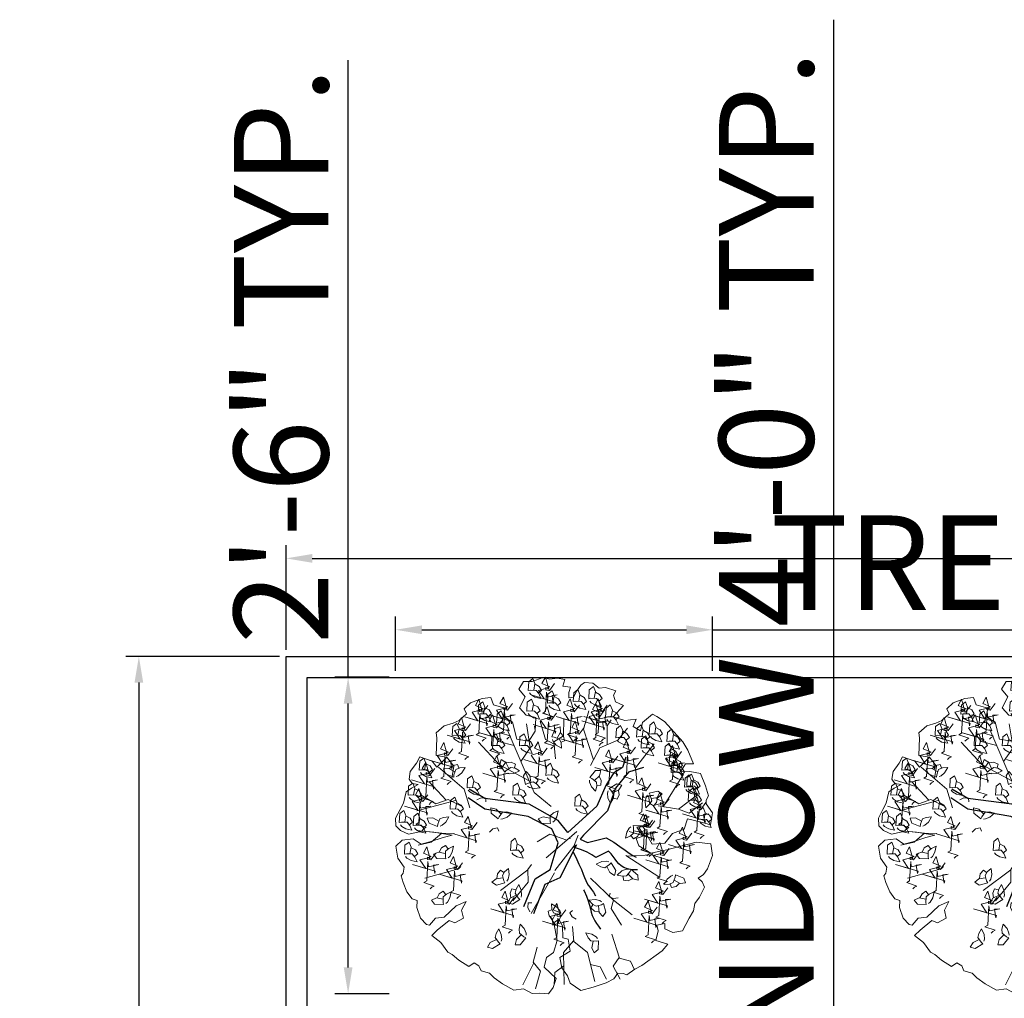
# Model space of a CAD drawing. Units: inches. Extents: x 2831 to 4250, y 1103 to 1797.
# Tile 4 of 15: x 3418 to 3512, y 1690 to 1783. Entities that reach past the tile are written whole.
import ezdxf

# ---------------------------------------------------------------- set-up
doc = ezdxf.new("R2010")
doc.units = ezdxf.units.IN
for name, color, linetype, lineweight in [('A-ANNO-DIMS', 2, 'Continuous', 18), ('ARBOL', 30, 'Continuous', 13), ('C-PROP', 7, 'Continuous', 25)]:
    doc.layers.add(name, color=color, linetype=linetype, lineweight=lineweight)
doc.layers.add('TALLO', color=36, linetype='Continuous')
doc.styles.get("Standard").update_dxf_attribs({"font": 'arial.ttf'})
doc.dimstyles.new('ISO-25', dxfattribs={"dimtxt": 9, "dimasz": 2.5, "dimexe": 1.25, "dimexo": 0.625, "dimtad": 1, "dimdec": 1, "dimlunit": 3, "dimtxsty": 'Standard', "dimcen": 2.5, "dimadec": 0, "dimazin": 0, "dimtfac": 1, "dimtdec": 1, "dimtmove": 0, "dimatfit": 3, "dimfxl": 1, "dimarcsym": 0})

# ---------------------------------------------------------------- blocks, each defined once
blk = doc.blocks.new('*D5')
at = {"layer": 'A-ANNO-DIMS', "color": 0, "lineweight": -2, "transparency": 16777216}
for p, q in [((3443.227, 1723.138), (3443.227, 1733.099)), ((3803.227, 1723.138), (3803.227, 1733.099)), ((3445.727, 1731.849), (3800.727, 1731.849))]:
    blk.add_line(p, q, dxfattribs=at)
at = {"layer": 'A-ANNO-DIMS', "color": 0, "transparency": 16777216}
for points in [[(3445.727, 1732.265), (3445.727, 1731.432), (3443.227, 1731.849)], [(3800.727, 1732.265), (3800.727, 1731.432), (3803.227, 1731.849)]]:
    blk.add_solid(points, dxfattribs=at)
at = {"layer": 'Defpoints', "color": 0, "transparency": 16777216}
for p in [(3803.227, 1731.849), (3443.227, 1722.513), (3803.227, 1722.513)]:
    blk.add_point(p, dxfattribs=at)
at = {"layer": 'A-ANNO-DIMS', "color": 0, "transparency": 16777216, "insert": (3623.227, 1737.072), "char_height": 9, "attachment_point": 5}
blk.add_mtext("30'", dxfattribs=at)
blk = doc.blocks.new('*D6')
at = {"layer": 'A-ANNO-DIMS', "color": 0, "lineweight": -2, "transparency": 16777216}
for p, q in [((3442.602, 1722.513), (3427.958, 1722.513)), ((3429.208, 1720.013), (3429.208, 1245.013)), ((3442.602, 1242.513), (3427.958, 1242.513))]:
    blk.add_line(p, q, dxfattribs=at)
at = {"layer": 'A-ANNO-DIMS', "color": 0, "transparency": 16777216}
for points in [[(3428.791, 1720.013), (3429.625, 1720.013), (3429.208, 1722.513)], [(3428.791, 1245.013), (3429.625, 1245.013), (3429.208, 1242.513)]]:
    blk.add_solid(points, dxfattribs=at)
at = {"layer": 'Defpoints', "color": 0, "transparency": 16777216}
for p in [(3443.227, 1722.513), (3429.208, 1242.513), (3443.227, 1242.513)]:
    blk.add_point(p, dxfattribs=at)
at = {"layer": 'A-ANNO-DIMS', "color": 0, "transparency": 16777216, "insert": (3423.988, 1482.513), "char_height": 9, "attachment_point": 5, "rotation": 90}
blk.add_mtext("40'", dxfattribs=at)
blk = doc.blocks.new('fresno')
at = {"layer": 'ARBOL'}
for p, q in [((2.96, 0.991), (3.575, 1.984)), ((-3.638, 1.194), (-4.164, 1.76)), ((-1.151, -0.932), (-1.99, -1.556)), ((-0.974, -3.757), (-1.31, -4.423))]:
    blk.add_line(p, q, dxfattribs=at)
blk.add_lwpolyline([(0.823, 4.745), (0.566, 4.764), (0.459, 4.687), (0.336, 4.518), (0.233, 4.322), (0.087, 4.298), (0.091, 4.464), (0.14, 4.621), (-0.09, 4.659), (-0.033, 4.863), (-0.264, 4.901), (-0.483, 4.866), (-0.686, 4.924), (-1.021, 4.801), (-1.288, 4.8), (-1.431, 4.563), (-1.234, 4.327), (-1.406, 4), (-1.205, 3.778), (-0.909, 3.705), (-0.931, 3.283), (-1.122, 2.983), (-1.491, 3.043), (-1.619, 3.562), (-1.9, 3.727), (-1.851, 3.982), (-2.197, 4.084), (-2.278, 4.31), (-2.543, 4.283), (-2.896, 4.152), (-3.091, 3.971), (-3.022, 3.817), (-3.244, 3.617), (-3.424, 3.528), (-3.697, 3.455), (-3.946, 3.236), (-3.922, 3.09), (-3.94, 2.548), (-3.617, 2.495), (-3.927, 2.19), (-4.062, 2.379), (-4.443, 2.512), (-4.546, 2.316), (-4.73, 2.062), (-4.767, 1.832), (-4.671, 1.698), (-4.486, 1.667), (-4.693, 1.559), (-4.854, 1.444), (-4.934, 1.102), (-5.037, 0.905), (-5.175, 0.644), (-5.166, 0.406), (-5.024, 0.264), (-4.781, 0.153), (-4.363, 0.249), (-4.014, 0.215), (-3.783, 0.177), (-3.46, 0.124), (-3.733, 0.051), (-4.132, -0.073), (-4.404, -0.146), (-4.639, 0.011), (-4.977, -0.028), (-5.172, -0.209), (-5.113, -0.574), (-4.921, -0.843), (-4.951, -1.027), (-5.012, -1.112), (-4.95, -1.311), (-4.83, -1.592), (-4.676, -1.807), (-4.518, -1.856), (-4.529, -2.068), (-4.417, -2.394), (-4.236, -2.59), (-4.143, -2.605), (-3.967, -2.397), (-3.703, -2.37), (-3.339, -2.027), (-3.032, -1.889), (-3.169, -2.15), (-3.115, -2.396), (-3.376, -2.542), (-3.552, -2.466), (-3.909, -2.762), (-4.077, -2.924), (-3.804, -3.135), (-3.592, -3.43), (-3.461, -3.499), (-3.253, -3.676), (-2.953, -3.867), (-2.792, -3.752), (-2.642, -3.848), (-2.572, -4.001), (-2.323, -4.066), (-2.18, -4.208), (-1.926, -4.392), (-1.58, -4.591), (-1.288, -4.545), (-1.027, -4.683), (-0.788, -4.675), (-0.531, -4.693), (-0.382, -4.505), (-0.29, -4.236), (-0.66, -3.891), (-0.588, -3.595), (-0.374, -3.441), (-0.267, -3.079), (-0.368, -2.541), (-0.208, -2.426), (-0.099, -2.633), (-0.087, -2.991), (0.071, -3.04), (0.129, -3.405), (-0.185, -3.59), (-0.119, -3.909), (0.055, -4.151), (0.136, -4.377), (0.456, -4.596), (0.828, -4.491), (1.227, -4.368), (1.461, -4.241), (1.583, -4.071), (1.748, -4.075), (1.86, -4.117), (2.101, -3.944), (2.308, -3.836), (2.925, -3.393), (3.101, -3.185), (2.74, -3.078), (2.812, -2.782), (2.769, -2.61), (3.015, -2.555), (3.012, -2.721), (3.254, -2.832), (3.546, -2.785), (3.752, -2.393), (3.882, -2.177), (3.92, -1.947), (4.069, -1.758), (4.214, -1.451), (4.144, -1.297), (4.021, -1.182), (4.182, -1.067), (4.304, -0.897), (4.464, -0.497), (4.429, -0.279), (4.406, -0.133), (3.964, -0.083), (3.074, -0.315), (2.582, -0.424), (2.217, -0.197), (2.136, 0.029), (2.462, 0.141), (2.628, -0.147), (3.012, -0.116), (3.249, 0.177), (3.602, 0.308), (3.701, 0.623), (4.089, 0.535), (4.404, 0.436), (4.464, 0.805), (4.272, 1.074), (4.267, 1.193), (4.336, 1.324), (4.243, 1.623), (4.092, 2.003), (3.769, 2.057), (3.485, 2.056), (3.642, 2.291), (3.88, 2.299), (3.71, 2.706), (3.563, 2.967), (3.201, 3.358), (3.001, 3.581), (2.766, 3.738), (2.635, 3.807), (2.332, 3.549), (2.268, 3.299), (2.052, 3.429), (2.136, 3.652), (1.798, 3.613), (1.437, 3.72), (1.755, 4.071), (1.513, 4.182), (1.451, 4.381), (1.519, 4.512), (1.204, 4.611), (1.012, 4.596)], close=True, dxfattribs=at)
for points in [[(-1.104, 4.45), (-1.063, 4.399), (-0.939, 4.325), (-0.757, 4.285), (-0.82, 4.431), (-0.903, 4.527), (-1.075, 4.533), (-1.143, 4.521), (-1.126, 4.792), (-1.002, 4.891), (-0.939, 4.738), (-0.975, 4.535)], [(-0.346, 4.735), (-0.501, 4.528), (-0.605, 4.545), (-0.605, 4.614), (-0.519, 4.563), (-0.622, 4.925), (-0.726, 4.735), (-0.484, 4.632), (-0.622, 4.58), (-0.829, 4.528), (-0.657, 4.27), (-1.053, 4.39), (-0.363, 4.183), (-0.381, 4.114), (-0.415, 4.373), (-0.26, 4.39), (-0.57, 4.321), (-0.588, 4.476), (-0.622, 3.89), (-0.708, 3.839), (-0.398, 3.735), (-0.467, 3.701), (-0.519, 3.649)], [(-0.935, 4.717), (-0.809, 4.65), (-0.736, 4.529), (-0.824, 4.459)], [(-0.521, 4.069), (-0.48, 4.018), (-0.356, 3.944), (-0.174, 3.904), (-0.237, 4.051), (-0.32, 4.146), (-0.492, 4.152), (-0.56, 4.14), (-0.543, 4.411), (-0.419, 4.511), (-0.356, 4.357), (-0.392, 4.154)], [(0.263, 4.114), (0.304, 4.063), (0.429, 3.989), (0.611, 3.948), (0.547, 4.095), (0.465, 4.191), (0.293, 4.197), (0.225, 4.185), (0.242, 4.456), (0.366, 4.555), (0.428, 4.402), (0.393, 4.199)], [(0.734, 4.203), (0.775, 4.152), (0.9, 4.078), (1.082, 4.038), (1.018, 4.185), (0.936, 4.281), (0.763, 4.287), (0.696, 4.274), (0.712, 4.546), (0.837, 4.645), (0.899, 4.491), (0.863, 4.289)], [(-2.368, 4.073), (-2.523, 3.866), (-2.627, 3.883), (-2.627, 3.952), (-2.541, 3.9), (-2.644, 4.262), (-2.748, 4.073), (-2.506, 3.969), (-2.644, 3.918), (-2.851, 3.866), (-2.679, 3.607), (-3.075, 3.728), (-2.385, 3.521), (-2.403, 3.452), (-2.437, 3.711), (-2.282, 3.728), (-2.592, 3.659), (-2.61, 3.814), (-2.644, 3.228), (-2.73, 3.176), (-2.42, 3.073), (-2.489, 3.038), (-2.541, 2.987)], [(-1.623, 4.132), (-1.778, 3.925), (-1.882, 3.942), (-1.882, 4.011), (-1.795, 3.959), (-1.899, 4.321), (-2.002, 4.132), (-1.761, 4.028), (-1.899, 3.977), (-2.106, 3.925), (-1.933, 3.666), (-2.33, 3.787), (-1.64, 3.58), (-1.657, 3.511), (-1.692, 3.77), (-1.537, 3.787), (-1.847, 3.718), (-1.864, 3.873), (-1.899, 3.287), (-1.985, 3.235), (-1.675, 3.132), (-1.744, 3.097), (-1.795, 3.046)], [(-1.149, 3.822), (-1.108, 3.771), (-0.983, 3.697), (-0.802, 3.657), (-0.865, 3.804), (-0.948, 3.9), (-1.12, 3.906), (-1.188, 3.893), (-1.171, 4.165), (-1.047, 4.264), (-0.984, 4.111), (-1.02, 3.908)], [(-0.352, 4.337), (-0.226, 4.269), (-0.153, 4.148), (-0.241, 4.078)], [(0.413, 4.08), (0.258, 3.873), (0.154, 3.89), (0.154, 3.959), (0.241, 3.908), (0.137, 4.27), (0.034, 4.08), (0.275, 3.977), (0.137, 3.925), (-0.07, 3.873), (0.103, 3.614), (-0.294, 3.735), (0.396, 3.528), (0.379, 3.459), (0.344, 3.718), (0.499, 3.735), (0.189, 3.666), (0.172, 3.821), (0.137, 3.235), (0.051, 3.183), (0.361, 3.08), (0.292, 3.046), (0.241, 2.994)], [(0.433, 4.381), (0.558, 4.314), (0.631, 4.193), (0.544, 4.122)], [(1.259, 4.08), (1.103, 3.873), (1, 3.89), (1, 3.959), (1.086, 3.908), (0.982, 4.27), (0.879, 4.08), (1.12, 3.977), (0.982, 3.925), (0.775, 3.873), (0.948, 3.614), (0.551, 3.735), (1.241, 3.528), (1.224, 3.459), (1.189, 3.718), (1.345, 3.735), (1.034, 3.666), (1.017, 3.821), (0.982, 3.235), (0.896, 3.183), (1.207, 3.08), (1.138, 3.046), (1.086, 2.994)], [(0.904, 4.471), (1.029, 4.404), (1.102, 4.282), (1.015, 4.212)], [(-2.629, 3.733), (-2.588, 3.682), (-2.463, 3.608), (-2.281, 3.568), (-2.345, 3.715), (-2.427, 3.81), (-2.6, 3.816), (-2.667, 3.804), (-2.651, 4.075), (-2.526, 4.175), (-2.464, 4.021), (-2.5, 3.818)], [(-2.459, 4), (-2.334, 3.933), (-2.261, 3.812), (-2.348, 3.742)], [(-2.068, 3.464), (-2.027, 3.413), (-1.903, 3.339), (-1.721, 3.299), (-1.784, 3.446), (-1.867, 3.542), (-2.039, 3.547), (-2.107, 3.535), (-2.09, 3.806), (-1.966, 3.906), (-1.903, 3.752), (-1.939, 3.55)], [(-0.287, 3.833), (-0.442, 3.626), (-0.546, 3.643), (-0.546, 3.712), (-0.46, 3.661), (-0.563, 4.023), (-0.667, 3.833), (-0.425, 3.73), (-0.563, 3.678), (-0.77, 3.626), (-0.598, 3.367), (-0.995, 3.488), (-0.304, 3.281), (-0.322, 3.212), (-0.356, 3.471), (-0.201, 3.488), (-0.511, 3.419), (-0.529, 3.574), (-0.563, 2.988), (-0.649, 2.936), (-0.339, 2.833), (-0.408, 2.799), (-0.46, 2.747)], [(-0.98, 4.09), (-0.854, 4.023), (-0.781, 3.901), (-0.869, 3.831)], [(1.189, 3.942), (1.034, 3.735), (0.931, 3.752), (0.931, 3.821), (1.017, 3.77), (0.913, 4.132), (0.81, 3.942), (1.051, 3.839), (0.913, 3.787), (0.706, 3.735), (0.879, 3.477), (0.482, 3.597), (1.172, 3.39), (1.155, 3.321), (1.12, 3.58), (1.276, 3.597), (0.965, 3.528), (0.948, 3.683), (0.913, 3.097), (0.827, 3.046), (1.138, 2.942), (1.069, 2.908), (1.017, 2.856)], [(0.837, 2.414), (0.533, 3.352), (0.697, 3.906)], [(1.25, 3.643), (1.291, 3.592), (1.416, 3.518), (1.597, 3.478), (1.534, 3.625), (1.451, 3.721), (1.279, 3.727), (1.211, 3.714), (1.228, 3.985), (1.352, 4.085), (1.415, 3.931), (1.379, 3.729)], [(1.419, 3.911), (1.545, 3.844), (1.618, 3.722), (1.53, 3.652)], [(-2.898, 3.511), (-3.053, 3.304), (-3.157, 3.321), (-3.157, 3.39), (-3.071, 3.339), (-3.174, 3.701), (-3.278, 3.511), (-3.036, 3.408), (-3.174, 3.356), (-3.381, 3.304), (-3.209, 3.046), (-3.605, 3.166), (-2.915, 2.959), (-2.932, 2.89), (-2.967, 3.149), (-2.812, 3.166), (-3.122, 3.097), (-3.14, 3.253), (-3.174, 2.666), (-3.26, 2.615), (-2.95, 2.511), (-3.019, 2.477), (-3.071, 2.425)], [(-1.951, 3.597), (-2.106, 3.39), (-2.209, 3.408), (-2.209, 3.477), (-2.123, 3.425), (-2.227, 3.787), (-2.33, 3.597), (-2.089, 3.494), (-2.227, 3.442), (-2.434, 3.39), (-2.261, 3.132), (-2.658, 3.252), (-1.968, 3.046), (-1.985, 2.977), (-2.02, 3.235), (-1.864, 3.252), (-2.175, 3.183), (-2.192, 3.339), (-2.227, 2.752), (-2.313, 2.701), (-2.002, 2.597), (-2.071, 2.563), (-2.123, 2.511)], [(-1.899, 3.732), (-1.773, 3.664), (-1.7, 3.543), (-1.788, 3.473)], [(-0.358, 2.895), (-0.615, 3.037), (-0.783, 3.596)], [(-0.063, 3.671), (-0.069, 3.151), (-0.364, 2.965), (-0.319, 2.449)], [(1.259, 2.882), (1.254, 3.446), (1.381, 3.636)], [(-3.413, 3.083), (-3.373, 3.032), (-3.248, 2.958), (-3.066, 2.918), (-3.129, 3.065), (-3.212, 3.161), (-3.384, 3.167), (-3.452, 3.154), (-3.435, 3.425), (-3.311, 3.525), (-3.248, 3.371), (-3.284, 3.169)], [(-3.244, 3.351), (-3.118, 3.284), (-3.045, 3.162), (-3.133, 3.092)], [(-0.448, 1), (-0.961, 1.419), (-1.784, 3.341)], [(-1.367, 2.367), (-1.081, 2.78), (-1.193, 3.514)], [(-0.923, 3.449), (-0.951, 3.425), (-0.93, 3.313)], [(-0.41, 3.035), (-0.387, 2.974), (-0.291, 2.865), (-0.131, 2.771), (-0.146, 2.93), (-0.195, 3.047), (-0.357, 3.106), (-0.425, 3.115), (-0.325, 3.368), (-0.176, 3.424), (-0.164, 3.258), (-0.261, 3.077)], [(0.558, 3.402), (0.403, 3.195), (0.299, 3.212), (0.299, 3.281), (0.386, 3.23), (0.282, 3.592), (0.179, 3.402), (0.42, 3.299), (0.282, 3.247), (0.075, 3.195), (0.248, 2.936), (-0.149, 3.057), (0.541, 2.85), (0.524, 2.781), (0.489, 3.04), (0.644, 3.057), (0.334, 2.988), (0.317, 3.143), (0.282, 2.557), (0.196, 2.505), (0.506, 2.402), (0.437, 2.368), (0.386, 2.316)], [(0.746, 2.242), (1.034, 2.786), (1.584, 3.019), (1.879, 3.374)], [(1.564, 3.016), (1.605, 2.965), (1.729, 2.891), (1.911, 2.851), (1.848, 2.998), (1.765, 3.094), (1.593, 3.099), (1.525, 3.087), (1.542, 3.358), (1.666, 3.458), (1.729, 3.304), (1.693, 3.102)], [(2.191, 3.038), (2.232, 2.987), (2.357, 2.913), (2.539, 2.873), (2.475, 3.02), (2.393, 3.116), (2.221, 3.122), (2.153, 3.109), (2.17, 3.381), (2.294, 3.48), (2.356, 3.326), (2.321, 3.124)], [(2.361, 3.306), (2.486, 3.239), (2.559, 3.117), (2.472, 3.047)], [(2.573, 3.128), (2.613, 3.077), (2.738, 3.003), (2.92, 2.963), (2.857, 3.11), (2.774, 3.205), (2.602, 3.211), (2.534, 3.199), (2.551, 3.47), (2.675, 3.57), (2.738, 3.416), (2.702, 3.214)], [(2.742, 3.396), (2.868, 3.328), (2.941, 3.207), (2.853, 3.137)], [(3.111, 2.904), (3.152, 2.853), (3.276, 2.779), (3.458, 2.739), (3.395, 2.886), (3.312, 2.981), (3.14, 2.987), (3.072, 2.975), (3.089, 3.246), (3.213, 3.346), (3.276, 3.192), (3.24, 2.99)], [(-2.225, 2.77), (-2.184, 2.718), (-2.06, 2.645), (-1.878, 2.604), (-1.941, 2.751), (-2.024, 2.847), (-2.196, 2.853), (-2.264, 2.84), (-2.247, 3.112), (-2.123, 3.211), (-2.06, 3.058), (-2.096, 2.855)], [(-1.575, 2.854), (-2.052, 2.969), (-2.2, 3.178)], [(-2.056, 3.037), (-1.93, 2.97), (-1.857, 2.849), (-1.945, 2.778)], [(-1.373, 2.77), (-1.332, 2.718), (-1.208, 2.645), (-1.026, 2.604), (-1.089, 2.751), (-1.172, 2.847), (-1.344, 2.853), (-1.412, 2.84), (-1.395, 3.112), (-1.271, 3.211), (-1.208, 3.058), (-1.244, 2.855)], [(-1.204, 3.037), (-1.078, 2.97), (-1.005, 2.849), (-1.093, 2.778)], [(-0.166, 3.238), (-0.068, 3.135), (-0.036, 2.997), (-0.141, 2.957)], [(1.733, 3.284), (1.859, 3.216), (1.932, 3.095), (1.844, 3.025)], [(2.326, 2.702), (2.367, 2.651), (2.492, 2.577), (2.673, 2.537), (2.61, 2.684), (2.527, 2.78), (2.355, 2.786), (2.287, 2.773), (2.304, 3.045), (2.428, 3.144), (2.491, 2.99), (2.455, 2.788)], [(3.28, 3.172), (3.406, 3.104), (3.479, 2.983), (3.391, 2.913)], [(-3.434, 2.752), (-3.59, 2.546), (-3.693, 2.563), (-3.693, 2.632), (-3.607, 2.58), (-3.71, 2.942), (-3.814, 2.752), (-3.572, 2.649), (-3.71, 2.597), (-3.917, 2.546), (-3.745, 2.287), (-4.142, 2.408), (-3.452, 2.201), (-3.469, 2.132), (-3.503, 2.39), (-3.348, 2.408), (-3.659, 2.339), (-3.676, 2.494), (-3.71, 1.908), (-3.797, 1.856), (-3.486, 1.753), (-3.555, 1.718), (-3.607, 1.666)], [(-1.112, 1.773), (-2.014, 2.265), (-2.654, 2.957)], [(-0.57, 2.77), (-0.726, 2.563), (-0.829, 2.58), (-0.829, 2.649), (-0.743, 2.597), (-0.846, 2.959), (-0.95, 2.77), (-0.708, 2.666), (-0.846, 2.615), (-1.053, 2.563), (-0.881, 2.304), (-1.278, 2.425), (-0.588, 2.218), (-0.605, 2.149), (-0.639, 2.408), (-0.484, 2.425), (-0.795, 2.356), (-0.812, 2.511), (-0.846, 1.925), (-0.933, 1.873), (-0.622, 1.77), (-0.691, 1.735), (-0.743, 1.684)], [(1.586, 2.528), (1.431, 2.321), (1.327, 2.339), (1.327, 2.408), (1.414, 2.356), (1.31, 2.718), (1.207, 2.528), (1.448, 2.425), (1.31, 2.373), (1.103, 2.321), (1.276, 2.063), (0.879, 2.184), (1.569, 1.977), (1.552, 1.908), (1.517, 2.166), (1.673, 2.184), (1.362, 2.115), (1.345, 2.27), (1.31, 1.684), (1.224, 1.632), (1.535, 1.528), (1.466, 1.494), (1.414, 1.442)], [(2.121, 2.804), (1.966, 2.597), (1.862, 2.615), (1.862, 2.683), (1.949, 2.632), (1.845, 2.994), (1.742, 2.804), (1.983, 2.701), (1.845, 2.649), (1.638, 2.597), (1.811, 2.339), (1.414, 2.459), (2.104, 2.252), (2.087, 2.184), (2.052, 2.442), (2.207, 2.459), (1.897, 2.39), (1.88, 2.546), (1.845, 1.959), (1.759, 1.908), (2.069, 1.804), (2, 1.77), (1.949, 1.718)], [(2.171, 1.674), (2.121, 2.172), (2.689, 2.898)], [(2.495, 2.97), (2.621, 2.903), (2.694, 2.781), (2.606, 2.711)], [(3.519, 2.666), (3.363, 2.459), (3.26, 2.477), (3.26, 2.546), (3.346, 2.494), (3.243, 2.856), (3.139, 2.666), (3.381, 2.563), (3.243, 2.511), (3.036, 2.459), (3.208, 2.201), (2.811, 2.321), (3.501, 2.115), (3.484, 2.046), (3.45, 2.304), (3.605, 2.321), (3.294, 2.252), (3.277, 2.408), (3.243, 1.821), (3.156, 1.77), (3.467, 1.666), (3.398, 1.632), (3.346, 1.58)], [(3.043, 2.478), (3.084, 2.427), (3.209, 2.353), (3.391, 2.313), (3.327, 2.46), (3.245, 2.556), (3.073, 2.562), (3.005, 2.549), (3.022, 2.82), (3.146, 2.92), (3.208, 2.766), (3.173, 2.564)], [(3.213, 2.746), (3.338, 2.679), (3.411, 2.557), (3.324, 2.487)], [(-4.422, 2.03), (-4.381, 1.979), (-4.257, 1.905), (-4.075, 1.865), (-4.138, 2.012), (-4.221, 2.108), (-4.393, 2.114), (-4.461, 2.101), (-4.444, 2.372), (-4.32, 2.472), (-4.257, 2.318), (-4.293, 2.116)], [(-3.468, 1.85), (-3.409, 2.222), (-3.628, 2.505)], [(-1.817, 2.351), (-1.972, 2.144), (-2.075, 2.162), (-2.075, 2.231), (-1.989, 2.179), (-2.093, 2.541), (-2.196, 2.351), (-1.955, 2.248), (-2.093, 2.196), (-2.3, 2.144), (-2.127, 1.886), (-2.524, 2.006), (-1.834, 1.8), (-1.851, 1.731), (-1.886, 1.989), (-1.73, 2.006), (-2.041, 1.937), (-2.058, 2.093), (-2.093, 1.506), (-2.179, 1.455), (-1.868, 1.351), (-1.937, 1.317), (-1.989, 1.265)], [(-1.786, 2.007), (-1.722, 1.99), (-1.578, 2.003), (-1.407, 2.078), (-1.545, 2.159), (-1.668, 2.188), (-1.811, 2.092), (-1.859, 2.042), (-2.004, 2.271), (-1.962, 2.425), (-1.821, 2.337), (-1.731, 2.152)], [(3.178, 2.165), (3.219, 2.113), (3.344, 2.04), (3.525, 1.999), (3.462, 2.146), (3.379, 2.242), (3.207, 2.248), (3.139, 2.236), (3.156, 2.507), (3.28, 2.606), (3.343, 2.453), (3.307, 2.25)], [(3.245, 1.963), (3.286, 1.912), (3.411, 1.838), (3.593, 1.798), (3.529, 1.945), (3.447, 2.041), (3.274, 2.046), (3.206, 2.034), (3.223, 2.305), (3.347, 2.405), (3.41, 2.251), (3.374, 2.049)], [(3.347, 2.432), (3.473, 2.365), (3.546, 2.244), (3.458, 2.173)], [(-3.986, 2.149), (-4.142, 1.942), (-4.245, 1.959), (-4.245, 2.028), (-4.159, 1.977), (-4.262, 2.339), (-4.366, 2.149), (-4.124, 2.046), (-4.262, 1.994), (-4.47, 1.942), (-4.297, 1.684), (-4.694, 1.804), (-4.004, 1.597), (-4.021, 1.528), (-4.055, 1.787), (-3.9, 1.804), (-4.211, 1.735), (-4.228, 1.89), (-4.262, 1.304), (-4.349, 1.253), (-4.038, 1.149), (-4.107, 1.115), (-4.159, 1.063)], [(-4.253, 2.298), (-4.127, 2.231), (-4.054, 2.109), (-4.142, 2.039)], [(-2.916, 0.958), (-3.096, 1.528), (-3.871, 2.197)], [(-3.331, 1.905), (-3.269, 1.928), (-3.161, 2.024), (-3.066, 2.184), (-3.226, 2.169), (-3.342, 2.121), (-3.401, 1.958), (-3.41, 1.89), (-3.663, 1.99), (-3.719, 2.139), (-3.554, 2.151), (-3.372, 2.054)], [(-3.533, 2.149), (-3.43, 2.247), (-3.292, 2.279), (-3.252, 2.174)], [(-1.806, 2.323), (-1.665, 2.343), (-1.534, 2.287), (-1.564, 2.179)], [(-0.566, 1.873), (-0.525, 1.822), (-0.4, 1.748), (-0.219, 1.708), (-0.282, 1.855), (-0.365, 1.951), (-0.537, 1.957), (-0.605, 1.944), (-0.588, 2.216), (-0.464, 2.315), (-0.401, 2.162), (-0.437, 1.959)], [(-0.397, 2.141), (-0.271, 2.074), (-0.198, 1.952), (-0.286, 1.882)], [(3.415, 2.231), (3.54, 2.163), (3.613, 2.042), (3.525, 1.972)], [(-2.965, 1.493), (-2.924, 1.441), (-2.799, 1.368), (-2.618, 1.327), (-2.681, 1.474), (-2.764, 1.57), (-2.936, 1.576), (-3.004, 1.564), (-2.987, 1.835), (-2.863, 1.934), (-2.8, 1.781), (-2.836, 1.578)], [(-1.164, 1.612), (-1.109, 1.576), (-0.967, 1.544), (-0.782, 1.562), (-0.888, 1.682), (-0.996, 1.748), (-1.162, 1.7), (-1.222, 1.667), (-1.29, 1.93), (-1.203, 2.063), (-1.096, 1.937), (-1.067, 1.733)], [(-1.085, 1.919), (-0.945, 1.893), (-0.838, 1.801), (-0.9, 1.707)], [(0.72, 1.798), (0.723, 1.733), (0.781, 1.6), (0.904, 1.46), (0.939, 1.616), (0.929, 1.742), (0.793, 1.848), (0.73, 1.878), (0.904, 2.088), (1.062, 2.095), (1.023, 1.934), (0.875, 1.791)], [(1.014, 1.915), (1.077, 1.787), (1.064, 1.646), (0.952, 1.64)], [(2.587, 1.684), (2.432, 1.477), (2.328, 1.494), (2.328, 1.563), (2.414, 1.511), (2.311, 1.873), (2.207, 1.684), (2.449, 1.58), (2.311, 1.528), (2.104, 1.477), (2.276, 1.218), (1.88, 1.339), (2.57, 1.132), (2.552, 1.063), (2.518, 1.321), (2.673, 1.339), (2.363, 1.27), (2.345, 1.425), (2.311, 0.839), (2.225, 0.787), (2.535, 0.684), (2.466, 0.649), (2.414, 0.597)], [(3.649, 1.515), (3.69, 1.464), (3.814, 1.39), (3.996, 1.35), (3.933, 1.497), (3.85, 1.592), (3.678, 1.598), (3.61, 1.586), (3.627, 1.857), (3.751, 1.957), (3.814, 1.803), (3.778, 1.601)], [(3.716, 1.537), (3.757, 1.486), (3.882, 1.412), (4.063, 1.372), (4, 1.519), (3.917, 1.615), (3.745, 1.621), (3.677, 1.608), (3.694, 1.88), (3.818, 1.979), (3.881, 1.825), (3.845, 1.623)], [(3.885, 1.805), (4.011, 1.738), (4.084, 1.616), (3.996, 1.546)], [(-4.193, 1.356), (-4.349, 1.149), (-4.452, 1.166), (-4.452, 1.235), (-4.366, 1.184), (-4.469, 1.546), (-4.573, 1.356), (-4.331, 1.253), (-4.469, 1.201), (-4.677, 1.149), (-4.504, 0.89), (-4.901, 1.011), (-4.211, 0.804), (-4.228, 0.735), (-4.262, 0.994), (-4.107, 1.011), (-4.418, 0.942), (-4.435, 1.097), (-4.469, 0.511), (-4.556, 0.459), (-4.245, 0.356), (-4.314, 0.322), (-4.366, 0.27)], [(-4.759, 1.269), (-4.718, 1.217), (-4.593, 1.144), (-4.411, 1.103), (-4.475, 1.25), (-4.557, 1.346), (-4.729, 1.352), (-4.797, 1.339), (-4.78, 1.611), (-4.656, 1.71), (-4.594, 1.557), (-4.629, 1.354)], [(-4.589, 1.536), (-4.464, 1.469), (-4.391, 1.348), (-4.478, 1.277)], [(-2.796, 1.76), (-2.67, 1.693), (-2.597, 1.572), (-2.685, 1.501)], [(-1.575, 1.269), (-1.534, 1.217), (-1.409, 1.144), (-1.228, 1.103), (-1.291, 1.25), (-1.373, 1.346), (-1.546, 1.352), (-1.614, 1.339), (-1.597, 1.611), (-1.473, 1.71), (-1.41, 1.557), (-1.446, 1.354)], [(-1.406, 1.536), (-1.28, 1.469), (-1.207, 1.348), (-1.295, 1.277)], [(1.283, 1.469), (1.266, 1.405), (1.279, 1.261), (1.354, 1.09), (1.435, 1.228), (1.464, 1.351), (1.368, 1.494), (1.318, 1.542), (1.547, 1.687), (1.7, 1.645), (1.613, 1.504), (1.428, 1.414)], [(3.761, 1.112), (3.802, 1.061), (3.926, 0.987), (4.108, 0.947), (4.045, 1.093), (3.962, 1.189), (3.79, 1.195), (3.722, 1.183), (3.739, 1.454), (3.863, 1.553), (3.926, 1.4), (3.89, 1.197)], [(3.818, 1.783), (3.944, 1.715), (4.017, 1.594), (3.929, 1.524)], [(-3.192, 1.017), (-3.578, 1.215), (-3.949, 1.081), (-4.398, 1.339)], [(-3.481, 0.843), (-3.44, 0.792), (-3.315, 0.718), (-3.133, 0.678), (-3.197, 0.825), (-3.279, 0.92), (-3.451, 0.926), (-3.519, 0.914), (-3.502, 1.185), (-3.378, 1.285), (-3.316, 1.131), (-3.351, 0.928)], [(-2.703, 1.201), (-2.575, 1.263), (-2.433, 1.251), (-2.428, 1.139)], [(0.308, 0.933), (0.349, 0.881), (0.474, 0.807), (0.656, 0.767), (0.592, 0.914), (0.51, 1.01), (0.337, 1.016), (0.27, 1.003), (0.286, 1.275), (0.411, 1.374), (0.473, 1.221), (0.437, 1.018)], [(0.478, 1.2), (0.603, 1.133), (0.676, 1.011), (0.589, 0.941)], [(1.599, 1.489), (1.618, 1.348), (1.563, 1.217), (1.455, 1.247)], [(2.479, 1.34), (2.443, 1.285), (2.411, 1.143), (2.429, 0.958), (2.549, 1.064), (2.615, 1.172), (2.567, 1.338), (2.534, 1.398), (2.797, 1.466), (2.93, 1.379), (2.804, 1.272), (2.6, 1.243)], [(3.139, 1.235), (2.984, 1.028), (2.88, 1.046), (2.88, 1.115), (2.967, 1.063), (2.863, 1.425), (2.759, 1.235), (3.001, 1.132), (2.863, 1.08), (2.656, 1.028), (2.828, 0.77), (2.432, 0.891), (3.122, 0.684), (3.105, 0.615), (3.07, 0.873), (3.225, 0.891), (2.915, 0.822), (2.897, 0.977), (2.863, 0.391), (2.777, 0.339), (3.087, 0.235), (3.018, 0.201), (2.967, 0.149)], [(2.786, 1.261), (2.76, 1.121), (2.668, 1.014), (2.574, 1.076)], [(4.01, 1.36), (3.422, 0.918)], [(4.26, 1.115), (4.105, 0.908), (4.002, 0.925), (4.002, 0.994), (4.088, 0.942), (3.984, 1.304), (3.881, 1.115), (4.122, 1.011), (3.984, 0.959), (3.777, 0.908), (3.95, 0.649), (3.553, 0.77), (4.243, 0.563), (4.226, 0.494), (4.191, 0.753), (4.347, 0.77), (4.036, 0.701), (4.019, 0.856), (3.984, 0.27), (3.898, 0.218), (4.209, 0.115), (4.14, 0.08), (4.088, 0.029)], [(3.93, 1.379), (4.056, 1.312), (4.129, 1.191), (4.041, 1.121)], [(-3.354, 1.176), (-4.529, 0.864)], [(-3.311, 1.111), (-3.186, 1.043), (-3.113, 0.922), (-3.2, 0.852)], [(-1.981, 0.615), (-1.915, 0.618), (-1.782, 0.676), (-1.643, 0.799), (-1.799, 0.834), (-1.925, 0.824), (-2.031, 0.688), (-2.061, 0.626), (-2.27, 0.799), (-2.278, 0.958), (-2.117, 0.918), (-1.974, 0.77)], [(2.808, 1.015), (3.422, 0.918), (3.422, 0.918), (3.748, 0.794), (4.154, 1.111)], [(4.075, 0.529), (4.116, 0.478), (4.24, 0.404), (4.422, 0.364), (4.359, 0.511), (4.276, 0.607), (4.104, 0.613), (4.036, 0.6), (4.053, 0.871), (4.177, 0.971), (4.24, 0.817), (4.204, 0.615)], [(-5.028, 0.44), (-4.987, 0.388), (-4.862, 0.315), (-4.68, 0.274), (-4.744, 0.421), (-4.826, 0.517), (-4.998, 0.523), (-5.066, 0.511), (-5.049, 0.782), (-4.925, 0.881), (-4.863, 0.728), (-4.898, 0.525)], [(-4.858, 0.707), (-4.733, 0.64), (-4.66, 0.519), (-4.747, 0.448)], [(-4.602, 0.35), (-4.561, 0.299), (-4.436, 0.225), (-4.254, 0.185), (-4.318, 0.332), (-4.4, 0.428), (-4.572, 0.433), (-4.64, 0.421), (-4.623, 0.692), (-4.499, 0.792), (-4.437, 0.638), (-4.472, 0.436)], [(-4.432, 0.618), (-4.307, 0.55), (-4.234, 0.429), (-4.321, 0.359)], [(-3.824, 0.404), (-3.763, 0.427), (-3.654, 0.523), (-3.559, 0.683), (-3.719, 0.668), (-3.835, 0.62), (-3.894, 0.457), (-3.903, 0.389), (-4.156, 0.489), (-4.212, 0.638), (-4.047, 0.65), (-3.865, 0.553)], [(-2.698, 0.509), (-2.854, 0.302), (-2.957, 0.319), (-2.957, 0.388), (-2.871, 0.336), (-2.974, 0.698), (-3.078, 0.509), (-2.836, 0.405), (-2.974, 0.353), (-3.182, 0.302), (-3.009, 0.043), (-3.406, 0.164), (-2.716, -0.043), (-2.733, -0.112), (-2.767, 0.147), (-2.612, 0.164), (-2.923, 0.095), (-2.94, 0.25), (-2.974, -0.336), (-3.061, -0.388), (-2.75, -0.491), (-2.819, -0.526), (-2.871, -0.577)], [(-0.397, 0.517), (-0.346, 0.557), (-0.272, 0.682), (-0.232, 0.864), (-0.379, 0.801), (-0.474, 0.718), (-0.48, 0.546), (-0.468, 0.478), (-0.739, 0.495), (-0.838, 0.619), (-0.685, 0.682), (-0.482, 0.646)], [(2.639, 0.58), (2.483, 0.373), (2.38, 0.391), (2.38, 0.46), (2.466, 0.408), (2.363, 0.77), (2.259, 0.58), (2.501, 0.477), (2.363, 0.425), (2.156, 0.373), (2.328, 0.115), (1.931, 0.235), (2.621, 0.029), (2.604, -0.04), (2.57, 0.218), (2.725, 0.235), (2.414, 0.166), (2.397, 0.322), (2.363, -0.265), (2.276, -0.316), (2.587, -0.42), (2.518, -0.454), (2.466, -0.506)], [(2.708, 0.563), (2.552, 0.356), (2.449, 0.373), (2.449, 0.442), (2.535, 0.391), (2.432, 0.753), (2.328, 0.563), (2.57, 0.46), (2.432, 0.408), (2.225, 0.356), (2.397, 0.097), (2, 0.218), (2.69, 0.011), (2.673, -0.058), (2.639, 0.201), (2.794, 0.218), (2.483, 0.149), (2.466, 0.304), (2.432, -0.282), (2.345, -0.334), (2.656, -0.437), (2.587, -0.471), (2.535, -0.523)], [(4.244, 0.797), (4.37, 0.73), (4.443, 0.608), (4.355, 0.538)], [(-2.322, 0.222), (-2.219, 0.321), (-2.081, 0.353), (-2.042, 0.248)], [(1.978, 0.384), (1.927, 0.343), (1.853, 0.218), (1.813, 0.036), (1.96, 0.1), (2.056, 0.182), (2.061, 0.355), (2.049, 0.422), (2.32, 0.406), (2.42, 0.281), (2.266, 0.219), (2.064, 0.254)], [(3.829, 0.184), (3.674, -0.023), (3.57, -0.006), (3.57, 0.063), (3.657, 0.011), (3.553, 0.373), (3.45, 0.184), (3.691, 0.08), (3.553, 0.029), (3.346, -0.023), (3.519, -0.282), (3.122, -0.161), (3.812, -0.368), (3.795, -0.437), (3.76, -0.178), (3.915, -0.161), (3.605, -0.23), (3.588, -0.075), (3.553, -0.661), (3.467, -0.713), (3.777, -0.816), (3.708, -0.851), (3.657, -0.902)], [(-3.394, 0.18), (-3.77, 0.182), (-4.532, 0.27)], [(-3.77, 0.182), (-4.09, -0.088), (-4.494, -0.18)], [(-1.642, -0.412), (-1.601, -0.463), (-1.477, -0.537), (-1.295, -0.577), (-1.358, -0.43), (-1.441, -0.334), (-1.613, -0.328), (-1.681, -0.341), (-1.664, -0.069), (-1.54, 0.03), (-1.477, -0.124), (-1.513, -0.326)], [(0.03, -0.026), (-0.491, 0.154), (-0.871, -0.08)], [(-0.596, -0.564), (0.03, -0.026), (0.339, 0.235)], [(0.38, 0.131), (0.248, -0.21), (-0.33, -0.951)], [(2.246, 0.214), (2.178, 0.089), (2.057, 0.016), (1.987, 0.103)], [(-4.871, -0.524), (-4.83, -0.575), (-4.705, -0.649), (-4.523, -0.689), (-4.587, -0.542), (-4.669, -0.446), (-4.841, -0.44), (-4.909, -0.453), (-4.893, -0.181), (-4.768, -0.082), (-4.706, -0.236), (-4.741, -0.438)], [(-4.701, -0.256), (-4.576, -0.323), (-4.503, -0.445), (-4.59, -0.515)], [(-3.952, -0.42), (-4.107, -0.627), (-4.211, -0.609), (-4.211, -0.54), (-4.124, -0.592), (-4.228, -0.23), (-4.331, -0.42), (-4.09, -0.523), (-4.228, -0.575), (-4.435, -0.627), (-4.262, -0.885), (-4.659, -0.765), (-3.969, -0.971), (-3.986, -1.04), (-4.021, -0.782), (-3.866, -0.765), (-4.176, -0.834), (-4.193, -0.678), (-4.228, -1.265), (-4.314, -1.316), (-4.004, -1.42), (-4.073, -1.454), (-4.124, -1.506)], [(-3.58, -0.559), (-3.529, -0.518), (-3.455, -0.393), (-3.415, -0.211), (-3.562, -0.275), (-3.658, -0.357), (-3.664, -0.53), (-3.651, -0.597), (-3.923, -0.581), (-4.022, -0.456), (-3.868, -0.394), (-3.666, -0.43)], [(-3.848, -0.389), (-3.781, -0.264), (-3.659, -0.191), (-3.589, -0.278)], [(-1.473, -0.144), (-1.347, -0.211), (-1.274, -0.333), (-1.362, -0.403)], [(3.139, -0.282), (2.984, -0.489), (2.88, -0.471), (2.88, -0.402), (2.967, -0.454), (2.863, -0.092), (2.759, -0.282), (3.001, -0.385), (2.863, -0.437), (2.656, -0.489), (2.828, -0.747), (2.432, -0.627), (3.122, -0.834), (3.105, -0.902), (3.07, -0.644), (3.225, -0.627), (2.915, -0.696), (2.897, -0.54), (2.863, -1.127), (2.777, -1.178), (3.087, -1.282), (3.018, -1.316), (2.967, -1.368)], [(-3.141, -0.713), (-3.296, -0.92), (-3.4, -0.902), (-3.4, -0.834), (-3.314, -0.885), (-3.417, -0.523), (-3.521, -0.713), (-3.279, -0.816), (-3.417, -0.868), (-3.624, -0.92), (-3.452, -1.178), (-3.848, -1.058), (-3.158, -1.265), (-3.175, -1.333), (-3.21, -1.075), (-3.055, -1.058), (-3.365, -1.127), (-3.383, -0.971), (-3.417, -1.558), (-3.503, -1.609), (-3.193, -1.713), (-3.262, -1.747), (-3.314, -1.799)], [(1.822, -0.495), (2.859, -1.165)], [(1.846, -0.51), (2.605, -0.469), (3.129, -0.637)], [(-3.195, -0.824), (-3.267, -0.898), (-4.285, -1.185)], [(-1.794, -1.268), (-1.758, -1.214), (-1.726, -1.072), (-1.744, -0.887), (-1.865, -0.993), (-1.93, -1.101), (-1.883, -1.266), (-1.85, -1.327), (-2.113, -1.395), (-2.246, -1.307), (-2.119, -1.2), (-1.916, -1.172)], [(-1.047, -0.767), (-1.151, -0.913), (-1.144, -1.307), (-1.61, -1.871)], [(1.304, -0.681), (1.241, -0.664), (1.097, -0.678), (0.926, -0.752), (1.064, -0.833), (1.187, -0.862), (1.33, -0.766), (1.377, -0.716), (1.523, -0.945), (1.481, -1.099), (1.34, -1.011), (1.25, -0.826)], [(-2.101, -1.19), (-2.076, -1.05), (-1.983, -0.943), (-1.889, -1.004)], [(-0.346, -1.024), (-1.05, -2.251)], [(0.748, -1.185), (1.452, -1.855), (2.021, -2.292)], [(1.903, -0.903), (1.837, -0.905), (1.704, -0.963), (1.565, -1.086), (1.721, -1.122), (1.847, -1.111), (1.953, -0.975), (1.983, -0.913), (2.192, -1.086), (2.2, -1.245), (2.039, -1.205), (1.896, -1.057)], [(2.02, -1.197), (1.891, -1.259), (1.75, -1.247), (1.745, -1.134)], [(3.253, -1.094), (3.192, -1.117), (3.083, -1.213), (2.988, -1.374), (3.148, -1.359), (3.264, -1.31), (3.323, -1.148), (3.332, -1.079), (3.585, -1.179), (3.641, -1.328), (3.476, -1.34), (3.294, -1.244)], [(-1.361, -1.756), (-1.343, -1.693), (-1.357, -1.548), (-1.431, -1.377), (-1.513, -1.515), (-1.542, -1.638), (-1.445, -1.781), (-1.395, -1.829), (-1.625, -1.974), (-1.778, -1.932), (-1.691, -1.791), (-1.506, -1.701)], [(3.105, -1.471), (2.949, -1.678), (2.846, -1.661), (2.846, -1.592), (2.932, -1.644), (2.829, -1.282), (2.725, -1.471), (2.967, -1.575), (2.829, -1.627), (2.621, -1.678), (2.794, -1.937), (2.397, -1.816), (3.087, -2.023), (3.07, -2.092), (3.036, -1.833), (3.191, -1.816), (2.88, -1.885), (2.863, -1.73), (2.829, -2.316), (2.742, -2.368), (3.053, -2.471), (2.984, -2.506), (2.932, -2.558)], [(3.455, -1.338), (3.352, -1.437), (3.214, -1.469), (3.175, -1.364)], [(-3.648, -1.948), (-3.596, -1.907), (-3.523, -1.782), (-3.482, -1.6), (-3.629, -1.664), (-3.725, -1.746), (-3.731, -1.919), (-3.719, -1.986), (-3.99, -1.97), (-4.089, -1.845), (-3.936, -1.783), (-3.733, -1.819)], [(-3.915, -1.778), (-3.848, -1.653), (-3.727, -1.58), (-3.656, -1.667)], [(-1.571, -1.764), (-1.726, -1.971), (-1.83, -1.954), (-1.83, -1.885), (-1.744, -1.937), (-1.847, -1.575), (-1.951, -1.764), (-1.709, -1.868), (-1.847, -1.92), (-2.054, -1.971), (-1.882, -2.23), (-2.278, -2.109), (-1.588, -2.316), (-1.605, -2.385), (-1.64, -2.127), (-1.485, -2.109), (-1.795, -2.178), (-1.813, -2.023), (-1.847, -2.609), (-1.933, -2.661), (-1.623, -2.764), (-1.692, -2.799), (-1.744, -2.851)], [(-1.677, -1.776), (-1.696, -1.635), (-1.641, -1.504), (-1.533, -1.534)], [(1.593, -1.781), (1.452, -1.801), (1.322, -1.746), (1.352, -1.637)], [(-1.092, -2.202), (-1.154, -2.074), (-1.142, -1.933), (-1.03, -1.928)], [(-0.001, -2.144), (-0.156, -2.351), (-0.26, -2.333), (-0.26, -2.264), (-0.174, -2.316), (-0.277, -1.954), (-0.381, -2.144), (-0.139, -2.247), (-0.277, -2.299), (-0.484, -2.351), (-0.312, -2.609), (-0.708, -2.489), (-0.018, -2.695), (-0.035, -2.764), (-0.07, -2.506), (0.085, -2.489), (-0.225, -2.558), (-0.243, -2.402), (-0.277, -2.989), (-0.363, -3.04), (-0.053, -3.144), (-0.122, -3.178), (-0.174, -3.23)], [(-0.161, -2.225), (-0.184, -2.163), (-0.28, -2.055), (-0.44, -1.96), (-0.425, -2.12), (-0.376, -2.236), (-0.214, -2.295), (-0.146, -2.304), (-0.246, -2.557), (-0.395, -2.613), (-0.407, -2.448), (-0.31, -2.266)], [(1.086, -1.899), (1.031, -1.863), (0.89, -1.831), (0.704, -1.849), (0.81, -1.969), (0.918, -2.035), (1.084, -1.987), (1.145, -1.954), (1.212, -2.218), (1.125, -2.35), (1.018, -2.224), (0.989, -2.02)], [(1.007, -2.206), (0.867, -2.181), (0.76, -2.088), (0.822, -1.994)], [(1.452, -1.855), (1.379, -2.105), (1.698, -2.609)], [(2.777, -2.058), (2.621, -2.264), (2.518, -2.247), (2.518, -2.178), (2.604, -2.23), (2.501, -1.868), (2.397, -2.058), (2.639, -2.161), (2.501, -2.213), (2.294, -2.264), (2.466, -2.523), (2.069, -2.402), (2.759, -2.609), (2.742, -2.678), (2.708, -2.42), (2.863, -2.402), (2.552, -2.471), (2.535, -2.316), (2.501, -2.902), (2.414, -2.954), (2.725, -3.057), (2.656, -3.092), (2.604, -3.144)], [(-0.405, -2.427), (-0.503, -2.324), (-0.535, -2.186), (-0.43, -2.146)], [(0.319, -2.428), (0.193, -2.361), (0.12, -2.239), (0.208, -2.169)], [(-1.201, -2.914), (-1.204, -2.849), (-1.262, -2.716), (-1.385, -2.576), (-1.42, -2.732), (-1.41, -2.858), (-1.274, -2.964), (-1.212, -2.994), (-1.385, -3.204), (-1.544, -3.211), (-1.504, -3.05), (-1.356, -2.907)], [(0.201, -2.655), (0.24, -3.105), (0.657, -3.436), (0.886, -4.322)], [(-1.966, -3.1), (-1.949, -3.037), (-1.962, -2.892), (-2.037, -2.722), (-2.118, -2.859), (-2.147, -2.982), (-2.051, -3.125), (-2.001, -3.173), (-2.23, -3.319), (-2.383, -3.277), (-2.296, -3.136), (-2.111, -3.046)], [(0.959, -3.012), (0.918, -2.961), (0.793, -2.887), (0.612, -2.847), (0.675, -2.994), (0.758, -3.089), (0.93, -3.095), (0.998, -3.083), (0.981, -3.354), (0.857, -3.453), (0.794, -3.3), (0.83, -3.097)], [(1.399, -2.886), (1.63, -3.612), (1.964, -3.708), (2.084, -3.964)], [(-0.923, -4.549), (-0.768, -4.012), (-0.99, -3.737), (-0.872, -3.28)], [(0.238, -3.084), (-0.067, -3.438), (-0.048, -4.412)], [(-0.059, -3.851), (-0.336, -4.054), (-0.355, -4.41)], [(0.752, -3.801), (1.042, -3.878), (1.233, -4.25)], [(1.625, -3.596), (1.438, -3.858), (1.657, -4.248)]]:
    blk.add_lwpolyline(points, dxfattribs=at)
for p in [(-0.308, 0.101), (0.124, 0.027)]:
    blk.add_point(p, dxfattribs=at)
at = {"layer": 'TALLO'}
for points in [[(1.829, 2.5), (1.722, 2.184), (1.454, 2.012), (1.213, 1.639), (0.944, 1.008), (0.06, 0.204), (-0.234, 0.577), (-1.119, 1.065), (-2.458, 1.237), (-2.941, 1.524)], [(2.364, 2.184), (1.909, 2.041), (1.507, 1.552), (1.266, 0.864), (0.542, 0.125), (0.433, 0.001), (0.662, -0.096), (1.228, 0.045), (1.455, -0.09), (1.644, -0.216), (1.8, -0.33), (1.931, -0.425), (2.042, -0.496), (2.141, -0.539)], [(-1.272, -2.047), (-0.931, -1.203), (-0.475, -0.916), (-0.234, -0.112), (-0.422, 0.318), (-1.146, 0.691), (-2.458, 0.921), (-2.967, 1.266)], [(2.177, -0.932), (2.008, -0.924), (1.873, -0.898), (1.766, -0.859), (1.682, -0.807), (1.613, -0.745), (1.554, -0.676), (1.499, -0.6), (1.442, -0.521), (1.376, -0.44), (1.298, -0.357), (0.908, -0.555), (0.791, -0.474), (0.647, -0.394), (0.474, -0.317), (0.265, -0.244), (0.226, -0.233), (0.328, -0.17), (-0.181, -1.175), (-0.637, -1.375), (-0.985, -2.265)], [(0.219, -0.386), (0.3, -0.544), (0.399, -0.753), (0.473, -0.922), (0.529, -1.057), (0.571, -1.164), (0.607, -1.251), (0.641, -1.324), (0.68, -1.389), (0.729, -1.454), (0.784, -1.525), (0.844, -1.61), (0.903, -1.717)], [(0.538, -1.536), (0.555, -1.568), (0.626, -1.728), (0.678, -1.871), (0.716, -2), (0.747, -2.115), (0.773, -2.219), (0.802, -2.314), (0.837, -2.401), (0.883, -2.483), (0.936, -2.562), (0.994, -2.642), (1.052, -2.727)]]:
    blk.add_lwpolyline(points, dxfattribs=at)
blk = doc.blocks.new('*D73')
at = {"layer": 'A-ANNO-DIMS', "color": 0, "lineweight": -2, "transparency": 16777216}
for p, q in [((3495.427, 1665.513), (3495.427, 1783.151)), ((3488.852, 1665.513), (3496.677, 1665.513)), ((3495.427, 1620.013), (3495.427, 1663.013)), ((3488.852, 1617.513), (3496.677, 1617.513))]:
    blk.add_line(p, q, dxfattribs=at)
at = {"layer": 'A-ANNO-DIMS', "color": 0, "transparency": 16777216}
for points in [[(3495.01, 1663.013), (3495.843, 1663.013), (3495.427, 1665.513)], [(3495.01, 1620.013), (3495.843, 1620.013), (3495.427, 1617.513)]]:
    blk.add_solid(points, dxfattribs=at)
at = {"layer": 'Defpoints', "color": 0, "transparency": 16777216}
for p in [(3488.227, 1665.513), (3495.427, 1665.513), (3488.227, 1617.513)]:
    blk.add_point(p, dxfattribs=at)
at = {"layer": 'A-ANNO-DIMS', "color": 0, "transparency": 16777216, "insert": (3490.145, 1725.582), "char_height": 9, "attachment_point": 5, "rotation": 90}
blk.add_mtext('WINDOW 4\'-0" TYP.', dxfattribs=at)
blk = doc.blocks.new('*D79')
at = {"layer": 'A-ANNO-DIMS', "color": 0, "lineweight": -2, "transparency": 16777216}
for p, q in [((3453.671, 1721.145), (3453.671, 1726.3)), ((3483.867, 1721.145), (3483.867, 1726.3)), ((3456.171, 1725.05), (3481.367, 1725.05)), ((3483.867, 1725.05), (3579.729, 1725.05))]:
    blk.add_line(p, q, dxfattribs=at)
at = {"layer": 'A-ANNO-DIMS', "color": 0, "transparency": 16777216}
for points in [[(3456.171, 1725.466), (3456.171, 1724.633), (3453.671, 1725.05)], [(3481.367, 1725.466), (3481.367, 1724.633), (3483.867, 1725.05)]]:
    blk.add_solid(points, dxfattribs=at)
at = {"layer": 'Defpoints', "color": 0, "transparency": 16777216}
for p in [(3483.867, 1725.05), (3453.671, 1720.52), (3483.867, 1720.52)]:
    blk.add_point(p, dxfattribs=at)
at = {"layer": 'A-ANNO-DIMS', "color": 0, "transparency": 16777216, "insert": (3533.048, 1730.27), "char_height": 9, "attachment_point": 5}
blk.add_mtext('TREE 2\'-6" TYP.', dxfattribs=at)
blk = doc.blocks.new('*D80')
at = {"layer": 'A-ANNO-DIMS', "color": 0, "lineweight": -2, "transparency": 16777216}
for p, q in [((3449.142, 1720.52), (3449.142, 1779.283)), ((3453.046, 1720.52), (3447.892, 1720.52)), ((3449.142, 1692.89), (3449.142, 1718.02)), ((3453.046, 1690.39), (3447.892, 1690.39))]:
    blk.add_line(p, q, dxfattribs=at)
at = {"layer": 'A-ANNO-DIMS', "color": 0, "transparency": 16777216}
for points in [[(3448.725, 1718.02), (3449.558, 1718.02), (3449.142, 1720.52)], [(3448.725, 1692.89), (3449.558, 1692.89), (3449.142, 1690.39)]]:
    blk.add_solid(points, dxfattribs=at)
at = {"layer": 'Defpoints', "color": 0, "transparency": 16777216}
for p in [(3449.142, 1720.52), (3453.671, 1720.52), (3453.671, 1690.39)]:
    blk.add_point(p, dxfattribs=at)
at = {"layer": 'A-ANNO-DIMS', "color": 0, "transparency": 16777216, "insert": (3443.922, 1751.152), "char_height": 9, "attachment_point": 5, "rotation": 90}
blk.add_mtext('2\'-6" TYP.', dxfattribs=at)

msp = doc.modelspace()

# ---------------------------------------------------------------- linework, layer by layer
at = {"layer": 'C-PROP'}
msp.add_lwpolyline([(3443.227, 1722.513), (3803.227, 1722.513), (3803.227, 1242.513), (3443.227, 1242.513)], close=True, dxfattribs=at)
msp.add_lwpolyline([(3445.227, 1244.513), (3445.227, 1720.513), (3801.227, 1720.513)], dxfattribs=at)

# ---------------------------------------------------------------- block references
at = {"layer": 'ARBOL', "xscale": 3.132679885015571, "yscale": 3.132679885015571, "zscale": 3.132679885015571}
for p in [(3469.882, 1705.093), (3515.869, 1705.093)]:
    msp.add_blockref('fresno', p, dxfattribs=at)

# ---------------------------------------------------------------- dimensions: what is measured, and where the dimension line sits
at = {"layer": 'A-ANNO-DIMS'}
for base, p1, p2, text, picture, middle in [((3495.427, 1665.513), (3488.227, 1617.513), (3488.227, 1665.513), 'WINDOW <> TYP.', '*D73', (3490.145, 1725.582)), ((3449.142, 1720.52), (3453.671, 1690.39), (3453.671, 1720.52), '<> TYP.', '*D80', (3443.922, 1751.152))]:
    dim = msp.add_linear_dim(base=base, p1=p1, p2=p2, angle=90, text=text, dimstyle='ISO-25', override={"dimdec": 1, "dimlfac": 1, "dimrnd": 0, "dimzin": 1, "dimdsep": 46, "dimlunit": 4, "dimfrac": 2}, dxfattribs=at)
    dim.commit()
    dim.dimension.update_dxf_attribs({"geometry": picture, "text_midpoint": middle})
dim = msp.add_linear_dim(base=(3483.867, 1725.05), p1=(3453.671, 1720.52), p2=(3483.867, 1720.52), text='TREE <> TYP.', dimstyle='ISO-25', override={"dimdec": 1, "dimlfac": 1, "dimrnd": 0, "dimzin": 1, "dimdsep": 46, "dimlunit": 4, "dimfrac": 2}, dxfattribs=at)
dim.commit()
dim.dimension.update_dxf_attribs({"geometry": '*D79', "text_midpoint": (3533.048, 1730.27)})
dim = msp.add_linear_dim(base=(3803.227, 1731.849), p1=(3443.227, 1722.513), p2=(3803.227, 1722.513), dimstyle='ISO-25', override={"dimclrd": 0, "dimclre": 0, "dimclrt": 0}, dxfattribs=at)
dim.commit()
dim.dimension.update_dxf_attribs({"geometry": '*D5', "text_midpoint": (3623.227, 1737.072)})
dim = msp.add_linear_dim(base=(3429.208, 1242.513), p1=(3443.227, 1722.513), p2=(3443.227, 1242.513), angle=90, dimstyle='ISO-25', override={"dimclrd": 0, "dimclre": 0, "dimclrt": 0}, dxfattribs=at)
dim.commit()
dim.dimension.update_dxf_attribs({"geometry": '*D6', "text_midpoint": (3423.988, 1482.513)})

doc.saveas('drawing.dxf')
